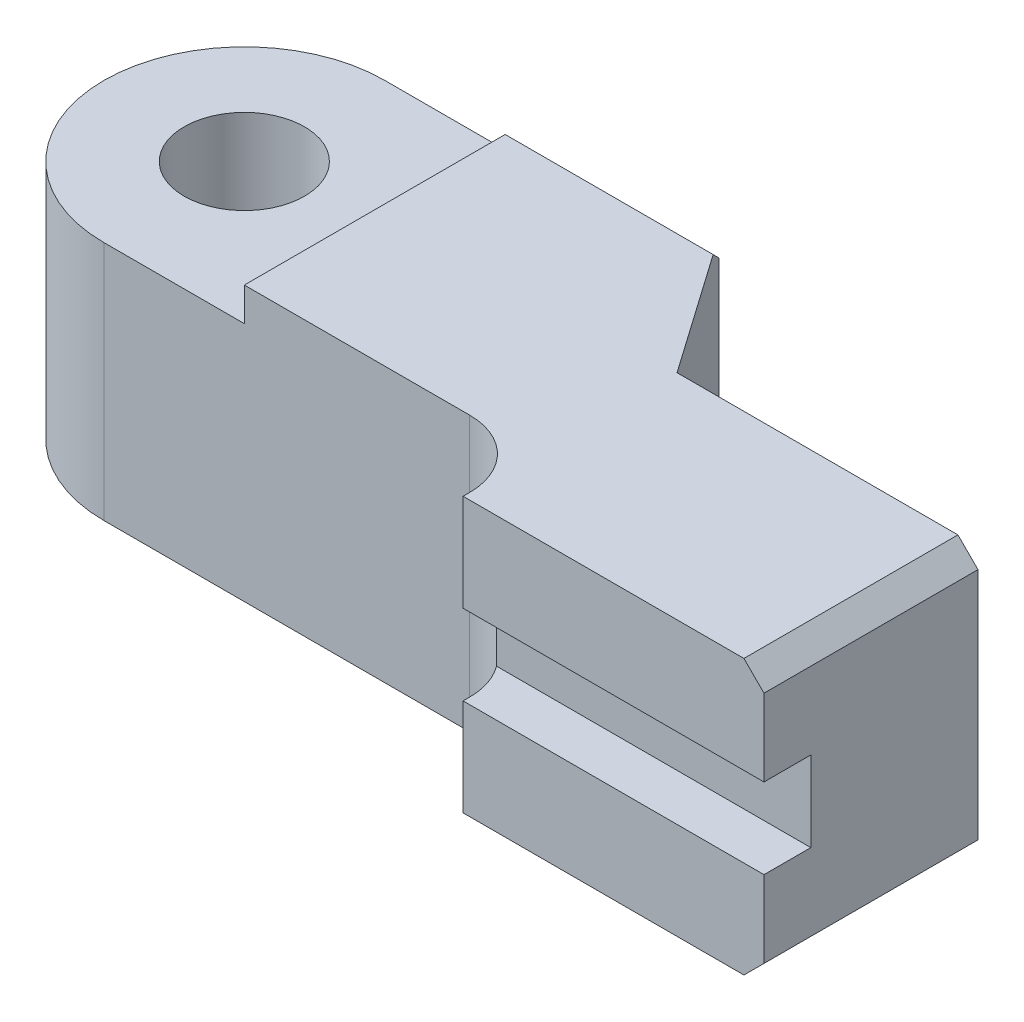
ISO-10303-21;
HEADER;
FILE_DESCRIPTION(('STEP AP214'),'2;1');
FILE_NAME('part.step','',(''),(''),'','','');
FILE_SCHEMA(('AUTOMOTIVE_DESIGN { 1 0 10303 214 1 1 1 1 }'));
ENDSEC;
DATA;
#1=APPLICATION_CONTEXT('core data for automotive mechanical design processes');
#2=APPLICATION_PROTOCOL_DEFINITION('international standard','automotive_design',2000,#1);
#3=PRODUCT_CONTEXT('',#1,'mechanical');
#4=PRODUCT('Part','Part','',(#3));
#5=PRODUCT_RELATED_PRODUCT_CATEGORY('part','',(#4));
#6=PRODUCT_DEFINITION_FORMATION('','',#4);
#7=PRODUCT_DEFINITION_CONTEXT('part definition',#1,'design');
#8=PRODUCT_DEFINITION('design','',#6,#7);
#9=PRODUCT_DEFINITION_SHAPE('','',#8);
#10=(LENGTH_UNIT() NAMED_UNIT(*) SI_UNIT(.MILLI.,.METRE.));
#11=(NAMED_UNIT(*) PLANE_ANGLE_UNIT() SI_UNIT($,.RADIAN.));
#12=(NAMED_UNIT(*) SI_UNIT($,.STERADIAN.) SOLID_ANGLE_UNIT());
#13=UNCERTAINTY_MEASURE_WITH_UNIT(LENGTH_MEASURE(1.E-05),#10,'distance_accuracy_value','');
#14=(GEOMETRIC_REPRESENTATION_CONTEXT(3) GLOBAL_UNCERTAINTY_ASSIGNED_CONTEXT((#13)) GLOBAL_UNIT_ASSIGNED_CONTEXT((#10,
#11,#12)) REPRESENTATION_CONTEXT('',''));
#15=CARTESIAN_POINT('',(0.,0.,0.));
#16=DIRECTION('',(0.,0.,1.));
#17=DIRECTION('',(1.,0.,0.));
#18=AXIS2_PLACEMENT_3D('',#15,#16,#17);
#19=CARTESIAN_POINT('',(54.7043583024038,20.5,0.));
#20=DIRECTION('',(-1.,0.,0.));
#21=DIRECTION('',(0.,0.,1.));
#22=AXIS2_PLACEMENT_3D('',#19,#20,#21);
#23=PLANE('',#22);
#24=DIRECTION('',(0.,-1.,0.));
#25=VECTOR('',#24,1.);
#26=CARTESIAN_POINT('',(54.7043583024038,20.5,32.));
#27=LINE('',#26,#25);
#28=CARTESIAN_POINT('',(54.7043583024038,-6.,32.));
#29=VERTEX_POINT('',#28);
#30=CARTESIAN_POINT('',(54.7043583024038,-17.5,32.));
#31=VERTEX_POINT('',#30);
#32=EDGE_CURVE('E243',#29,#31,#27,.T.);
#33=ORIENTED_EDGE('',*,*,#32,.T.);
#34=DIRECTION('',(0.,0.,-1.));
#35=VECTOR('',#34,1.);
#36=CARTESIAN_POINT('',(54.7043583024038,-17.5,0.));
#37=LINE('',#36,#35);
#38=CARTESIAN_POINT('',(54.7043583024038,-17.5,0.));
#39=VERTEX_POINT('',#38);
#40=EDGE_CURVE('E300',#31,#39,#37,.T.);
#41=ORIENTED_EDGE('',*,*,#40,.T.);
#42=DIRECTION('',(0.,-1.,0.));
#43=VECTOR('',#42,1.);
#44=CARTESIAN_POINT('',(54.7043583024038,20.5,0.));
#45=LINE('',#44,#43);
#46=CARTESIAN_POINT('',(54.7043583024038,17.5,0.));
#47=VERTEX_POINT('',#46);
#48=EDGE_CURVE('E288',#47,#39,#45,.T.);
#49=ORIENTED_EDGE('',*,*,#48,.F.);
#50=DIRECTION('',(0.,0.,1.));
#51=VECTOR('',#50,1.);
#52=CARTESIAN_POINT('',(54.7043583024038,17.5,32.));
#53=LINE('',#52,#51);
#54=CARTESIAN_POINT('',(54.7043583024038,17.5,32.));
#55=VERTEX_POINT('',#54);
#56=EDGE_CURVE('E299',#47,#55,#53,.T.);
#57=ORIENTED_EDGE('',*,*,#56,.T.);
#58=CARTESIAN_POINT('',(54.7043583024038,6.,32.));
#59=VERTEX_POINT('',#58);
#60=EDGE_CURVE('E194',#55,#59,#27,.T.);
#61=ORIENTED_EDGE('',*,*,#60,.T.);
#62=DIRECTION('',(0.,0.,1.));
#63=VECTOR('',#62,1.);
#64=CARTESIAN_POINT('',(54.7043583024038,6.,39.));
#65=LINE('',#64,#63);
#66=CARTESIAN_POINT('',(54.7043583024038,6.,25.));
#67=VERTEX_POINT('',#66);
#68=EDGE_CURVE('E175',#67,#59,#65,.T.);
#69=ORIENTED_EDGE('',*,*,#68,.F.);
#70=DIRECTION('',(0.,1.,0.));
#71=VECTOR('',#70,1.);
#72=CARTESIAN_POINT('',(54.7043583024038,6.,25.));
#73=LINE('',#72,#71);
#74=CARTESIAN_POINT('',(54.7043583024038,-6.,25.));
#75=VERTEX_POINT('',#74);
#76=EDGE_CURVE('E183',#75,#67,#73,.T.);
#77=ORIENTED_EDGE('',*,*,#76,.F.);
#78=DIRECTION('',(0.,0.,-1.));
#79=VECTOR('',#78,1.);
#80=CARTESIAN_POINT('',(54.7043583024038,-6.,39.));
#81=LINE('',#80,#79);
#82=EDGE_CURVE('E185',#29,#75,#81,.T.);
#83=ORIENTED_EDGE('',*,*,#82,.F.);
#84=EDGE_LOOP('',(#33,#41,#49,#57,#61,#69,#77,#83));
#85=FACE_BOUND('',#84,.T.);
#86=ADVANCED_FACE('F41',(#85),#23,.F.);
#87=CARTESIAN_POINT('',(9.70435830240385,20.5,31.0000000000001));
#88=DIRECTION('',(1.,0.,0.));
#89=DIRECTION('',(0.,0.,-1.));
#90=AXIS2_PLACEMENT_3D('',#87,#88,#89);
#91=PLANE('',#90);
#92=DIRECTION('',(0.,-1.,0.));
#93=VECTOR('',#92,1.);
#94=CARTESIAN_POINT('',(9.70435830240385,20.5,32.));
#95=LINE('',#94,#93);
#96=CARTESIAN_POINT('',(9.70435830240385,-6.,32.));
#97=VERTEX_POINT('',#96);
#98=CARTESIAN_POINT('',(9.70435830240385,-20.5,32.));
#99=VERTEX_POINT('',#98);
#100=EDGE_CURVE('E266',#97,#99,#95,.T.);
#101=ORIENTED_EDGE('',*,*,#100,.F.);
#102=DIRECTION('',(0.,0.,-1.));
#103=VECTOR('',#102,1.);
#104=CARTESIAN_POINT('',(9.70435830240385,-6.,31.0000000000001));
#105=LINE('',#104,#103);
#106=CARTESIAN_POINT('',(9.70435830240385,-6.,31.0000000000001));
#107=VERTEX_POINT('',#106);
#108=EDGE_CURVE('E201',#97,#107,#105,.T.);
#109=ORIENTED_EDGE('',*,*,#108,.T.);
#110=DIRECTION('',(0.,-1.,0.));
#111=VECTOR('',#110,1.);
#112=CARTESIAN_POINT('',(9.70435830240385,20.5,31.0000000000001));
#113=LINE('',#112,#111);
#114=CARTESIAN_POINT('',(9.70435830240385,-20.5,31.0000000000001));
#115=VERTEX_POINT('',#114);
#116=EDGE_CURVE('E269',#107,#115,#113,.T.);
#117=ORIENTED_EDGE('',*,*,#116,.T.);
#118=DIRECTION('',(0.,0.,1.));
#119=VECTOR('',#118,1.);
#120=CARTESIAN_POINT('',(9.70435830240385,-20.5,31.0000000000001));
#121=LINE('',#120,#119);
#122=EDGE_CURVE('E257',#115,#99,#121,.T.);
#123=ORIENTED_EDGE('',*,*,#122,.T.);
#124=EDGE_LOOP('',(#101,#109,#117,#123));
#125=FACE_BOUND('',#124,.T.);
#126=ADVANCED_FACE('F362',(#125),#91,.F.);
#127=CARTESIAN_POINT('',(9.70435830240385,20.5,32.));
#128=DIRECTION('',(0.,0.,-1.));
#129=DIRECTION('',(-1.,0.,0.));
#130=AXIS2_PLACEMENT_3D('',#127,#128,#129);
#131=PLANE('',#130);
#132=DIRECTION('',(1.,0.,0.));
#133=VECTOR('',#132,1.);
#134=CARTESIAN_POINT('',(9.70435830240385,-20.5,32.));
#135=LINE('',#134,#133);
#136=CARTESIAN_POINT('',(51.7043583024038,-20.5,32.));
#137=VERTEX_POINT('',#136);
#138=EDGE_CURVE('E235',#99,#137,#135,.T.);
#139=ORIENTED_EDGE('',*,*,#138,.T.);
#140=DIRECTION('',(-0.707106781186547,-0.707106781186548,0.));
#141=VECTOR('',#140,1.);
#142=CARTESIAN_POINT('',(54.7043583024038,-17.5,32.));
#143=LINE('',#142,#141);
#144=EDGE_CURVE('E310',#137,#31,#143,.F.);
#145=ORIENTED_EDGE('',*,*,#144,.T.);
#146=ORIENTED_EDGE('',*,*,#32,.F.);
#147=DIRECTION('',(-1.,0.,0.));
#148=VECTOR('',#147,1.);
#149=CARTESIAN_POINT('',(9.70435830240385,-6.,32.));
#150=LINE('',#149,#148);
#151=EDGE_CURVE('E291',#29,#97,#150,.T.);
#152=ORIENTED_EDGE('',*,*,#151,.T.);
#153=ORIENTED_EDGE('',*,*,#100,.T.);
#154=EDGE_LOOP('',(#139,#145,#146,#152,#153));
#155=FACE_BOUND('',#154,.T.);
#156=ADVANCED_FACE('F369',(#155),#131,.F.);
#157=CARTESIAN_POINT('',(-55.,20.5,21.));
#158=DIRECTION('',(0.,0.,-1.));
#159=DIRECTION('',(-1.,0.,0.));
#160=AXIS2_PLACEMENT_3D('',#157,#158,#159);
#161=PLANE('',#160);
#162=DIRECTION('',(1.,0.,0.));
#163=VECTOR('',#162,1.);
#164=CARTESIAN_POINT('',(-55.,15.5,21.));
#165=LINE('',#164,#163);
#166=CARTESIAN_POINT('',(-55.,15.5,21.));
#167=VERTEX_POINT('',#166);
#168=CARTESIAN_POINT('',(-34.,15.5,21.));
#169=VERTEX_POINT('',#168);
#170=EDGE_CURVE('E215',#167,#169,#165,.T.);
#171=ORIENTED_EDGE('',*,*,#170,.F.);
#172=DIRECTION('',(0.,-1.,0.));
#173=VECTOR('',#172,1.);
#174=CARTESIAN_POINT('',(-55.,20.5,21.));
#175=LINE('',#174,#173);
#176=CARTESIAN_POINT('',(-55.,-20.5,21.));
#177=VERTEX_POINT('',#176);
#178=EDGE_CURVE('E280',#167,#177,#175,.T.);
#179=ORIENTED_EDGE('',*,*,#178,.T.);
#180=DIRECTION('',(1.,0.,0.));
#181=VECTOR('',#180,1.);
#182=CARTESIAN_POINT('',(-55.,-20.5,21.));
#183=LINE('',#182,#181);
#184=CARTESIAN_POINT('',(-0.295641697596222,-20.5,21.));
#185=VERTEX_POINT('',#184);
#186=EDGE_CURVE('E254',#177,#185,#183,.T.);
#187=ORIENTED_EDGE('',*,*,#186,.T.);
#188=DIRECTION('',(0.,-1.,0.));
#189=VECTOR('',#188,1.);
#190=CARTESIAN_POINT('',(-0.295641697596222,20.5,21.));
#191=LINE('',#190,#189);
#192=CARTESIAN_POINT('',(-0.295641697596222,20.5,21.));
#193=VERTEX_POINT('',#192);
#194=EDGE_CURVE('E273',#193,#185,#191,.T.);
#195=ORIENTED_EDGE('',*,*,#194,.F.);
#196=DIRECTION('',(1.,0.,0.));
#197=VECTOR('',#196,1.);
#198=CARTESIAN_POINT('',(-55.,20.5,21.));
#199=LINE('',#198,#197);
#200=CARTESIAN_POINT('',(-34.,20.5,21.));
#201=VERTEX_POINT('',#200);
#202=EDGE_CURVE('E232',#201,#193,#199,.T.);
#203=ORIENTED_EDGE('',*,*,#202,.F.);
#204=DIRECTION('',(0.,1.,0.));
#205=VECTOR('',#204,1.);
#206=CARTESIAN_POINT('',(-34.,15.5,21.));
#207=LINE('',#206,#205);
#208=EDGE_CURVE('E218',#169,#201,#207,.T.);
#209=ORIENTED_EDGE('',*,*,#208,.F.);
#210=EDGE_LOOP('',(#171,#179,#187,#195,#203,#209));
#211=FACE_BOUND('',#210,.T.);
#212=ADVANCED_FACE('F425',(#211),#161,.F.);
#213=CARTESIAN_POINT('',(-55.,20.5,0.));
#214=DIRECTION('',(0.,-1.,0.));
#215=DIRECTION('',(0.,0.,-1.));
#216=AXIS2_PLACEMENT_3D('',#213,#214,#215);
#217=CYLINDRICAL_SURFACE('',#216,21.);
#218=CARTESIAN_POINT('',(-55.,15.5,0.));
#219=DIRECTION('',(0.,1.,0.));
#220=DIRECTION('',(0.,0.,1.));
#221=AXIS2_PLACEMENT_3D('',#218,#219,#220);
#222=CIRCLE('',#221,21.);
#223=CARTESIAN_POINT('',(-55.,15.5,-21.));
#224=VERTEX_POINT('',#223);
#225=EDGE_CURVE('E209',#224,#167,#222,.T.);
#226=ORIENTED_EDGE('',*,*,#225,.F.);
#227=DIRECTION('',(0.,-1.,0.));
#228=VECTOR('',#227,1.);
#229=CARTESIAN_POINT('',(-55.,20.5,-21.));
#230=LINE('',#229,#228);
#231=CARTESIAN_POINT('',(-55.,-20.5,-21.));
#232=VERTEX_POINT('',#231);
#233=EDGE_CURVE('E276',#224,#232,#230,.T.);
#234=ORIENTED_EDGE('',*,*,#233,.T.);
#235=CARTESIAN_POINT('',(-55.,-20.5,0.));
#236=DIRECTION('',(0.,1.,0.));
#237=DIRECTION('',(0.,0.,1.));
#238=AXIS2_PLACEMENT_3D('',#235,#236,#237);
#239=CIRCLE('',#238,21.);
#240=EDGE_CURVE('E252',#232,#177,#239,.T.);
#241=ORIENTED_EDGE('',*,*,#240,.T.);
#242=ORIENTED_EDGE('',*,*,#178,.F.);
#243=EDGE_LOOP('',(#226,#234,#241,#242));
#244=FACE_BOUND('',#243,.T.);
#245=ADVANCED_FACE('F407',(#244),#217,.T.);
#246=CARTESIAN_POINT('',(-55.,20.5,0.));
#247=DIRECTION('',(0.,-1.,0.));
#248=DIRECTION('',(0.,0.,-1.));
#249=AXIS2_PLACEMENT_3D('',#246,#247,#248);
#250=CYLINDRICAL_SURFACE('',#249,9.);
#251=CARTESIAN_POINT('',(-55.,-20.5,0.));
#252=DIRECTION('',(0.,1.,0.));
#253=DIRECTION('',(0.,0.,1.));
#254=AXIS2_PLACEMENT_3D('',#251,#252,#253);
#255=CIRCLE('',#254,9.);
#256=CARTESIAN_POINT('',(-55.,-20.5,8.99999999999999));
#257=VERTEX_POINT('',#256);
#258=EDGE_CURVE('E223',#257,#257,#255,.T.);
#259=ORIENTED_EDGE('',*,*,#258,.F.);
#260=EDGE_LOOP('',(#259));
#261=FACE_BOUND('',#260,.T.);
#262=CARTESIAN_POINT('',(-55.,15.5,0.));
#263=DIRECTION('',(0.,1.,0.));
#264=DIRECTION('',(0.,0.,1.));
#265=AXIS2_PLACEMENT_3D('',#262,#263,#264);
#266=CIRCLE('',#265,9.);
#267=CARTESIAN_POINT('',(-55.,15.5,8.99999999999999));
#268=VERTEX_POINT('',#267);
#269=EDGE_CURVE('E224',#268,#268,#266,.T.);
#270=ORIENTED_EDGE('',*,*,#269,.T.);
#271=EDGE_LOOP('',(#270));
#272=FACE_BOUND('',#271,.T.);
#273=ADVANCED_FACE('F404',(#261,#272),#250,.F.);
#274=CARTESIAN_POINT('',(-0.295641697596152,20.5,31.));
#275=DIRECTION('',(0.,1.,0.));
#276=DIRECTION('',(0.,0.,1.));
#277=AXIS2_PLACEMENT_3D('',#274,#275,#276);
#278=PLANE('',#277);
#279=DIRECTION('',(1.,0.,0.));
#280=VECTOR('',#279,1.);
#281=CARTESIAN_POINT('',(9.70435830240385,20.5,32.));
#282=LINE('',#281,#280);
#283=CARTESIAN_POINT('',(9.70435830240385,20.5,32.));
#284=VERTEX_POINT('',#283);
#285=CARTESIAN_POINT('',(51.7043583024039,20.5,32.));
#286=VERTEX_POINT('',#285);
#287=EDGE_CURVE('E241',#284,#286,#282,.T.);
#288=ORIENTED_EDGE('',*,*,#287,.T.);
#289=DIRECTION('',(0.,0.,-1.));
#290=VECTOR('',#289,1.);
#291=CARTESIAN_POINT('',(51.7043583024039,20.5,0.));
#292=LINE('',#291,#290);
#293=CARTESIAN_POINT('',(51.7043583024039,20.5,0.));
#294=VERTEX_POINT('',#293);
#295=EDGE_CURVE('E314',#286,#294,#292,.T.);
#296=ORIENTED_EDGE('',*,*,#295,.T.);
#297=DIRECTION('',(-1.,0.,0.));
#298=VECTOR('',#297,1.);
#299=CARTESIAN_POINT('',(54.7043583024038,20.5,0.));
#300=LINE('',#299,#298);
#301=CARTESIAN_POINT('',(9.70435830240384,20.5,0.));
#302=VERTEX_POINT('',#301);
#303=EDGE_CURVE('E228',#294,#302,#300,.T.);
#304=ORIENTED_EDGE('',*,*,#303,.T.);
#305=DIRECTION('',(-0.573576436351043,0.,-0.819152044288994));
#306=VECTOR('',#305,1.);
#307=CARTESIAN_POINT('',(-4.99999999999999,20.5,-21.0000000000001));
#308=LINE('',#307,#306);
#309=CARTESIAN_POINT('',(-2.89937738537089,20.5,-18.0000000000001));
#310=VERTEX_POINT('',#309);
#311=EDGE_CURVE('E233',#302,#310,#308,.T.);
#312=ORIENTED_EDGE('',*,*,#311,.T.);
#313=DIRECTION('',(-1.,0.,0.));
#314=VECTOR('',#313,1.);
#315=CARTESIAN_POINT('',(-34.,20.5,-18.));
#316=LINE('',#315,#314);
#317=CARTESIAN_POINT('',(-34.,20.5,-18.));
#318=VERTEX_POINT('',#317);
#319=EDGE_CURVE('E313',#310,#318,#316,.T.);
#320=ORIENTED_EDGE('',*,*,#319,.T.);
#321=DIRECTION('',(0.,0.,-1.));
#322=VECTOR('',#321,1.);
#323=CARTESIAN_POINT('',(-34.,20.5,-21.0000000000001));
#324=LINE('',#323,#322);
#325=EDGE_CURVE('E207',#201,#318,#324,.T.);
#326=ORIENTED_EDGE('',*,*,#325,.F.);
#327=ORIENTED_EDGE('',*,*,#202,.T.);
#328=CARTESIAN_POINT('',(-0.295641697596152,20.5,31.));
#329=DIRECTION('',(0.,-1.,0.));
#330=DIRECTION('',(0.,0.,1.));
#331=AXIS2_PLACEMENT_3D('',#328,#329,#330);
#332=CIRCLE('',#331,10.);
#333=CARTESIAN_POINT('',(9.70435830240385,20.5,31.0000000000001));
#334=VERTEX_POINT('',#333);
#335=EDGE_CURVE('E240',#193,#334,#332,.T.);
#336=ORIENTED_EDGE('',*,*,#335,.T.);
#337=DIRECTION('',(0.,0.,1.));
#338=VECTOR('',#337,1.);
#339=CARTESIAN_POINT('',(9.70435830240385,20.5,31.0000000000001));
#340=LINE('',#339,#338);
#341=EDGE_CURVE('E239',#334,#284,#340,.T.);
#342=ORIENTED_EDGE('',*,*,#341,.T.);
#343=EDGE_LOOP('',(#288,#296,#304,#312,#320,#326,#327,#336,#342));
#344=FACE_BOUND('',#343,.T.);
#345=ADVANCED_FACE('F330',(#344),#278,.T.);
#346=CARTESIAN_POINT('',(-0.295641697596152,-20.5,31.));
#347=DIRECTION('',(0.,1.,0.));
#348=DIRECTION('',(0.,0.,1.));
#349=AXIS2_PLACEMENT_3D('',#346,#347,#348);
#350=PLANE('',#349);
#351=DIRECTION('',(-1.,0.,0.));
#352=VECTOR('',#351,1.);
#353=CARTESIAN_POINT('',(54.7043583024038,-20.5,0.));
#354=LINE('',#353,#352);
#355=CARTESIAN_POINT('',(51.7043583024038,-20.5,0.));
#356=VERTEX_POINT('',#355);
#357=CARTESIAN_POINT('',(9.70435830240384,-20.5,0.));
#358=VERTEX_POINT('',#357);
#359=EDGE_CURVE('E229',#356,#358,#354,.T.);
#360=ORIENTED_EDGE('',*,*,#359,.F.);
#361=DIRECTION('',(0.,0.,1.));
#362=VECTOR('',#361,1.);
#363=CARTESIAN_POINT('',(51.7043583024039,-20.5,31.));
#364=LINE('',#363,#362);
#365=EDGE_CURVE('E307',#356,#137,#364,.T.);
#366=ORIENTED_EDGE('',*,*,#365,.T.);
#367=ORIENTED_EDGE('',*,*,#138,.F.);
#368=ORIENTED_EDGE('',*,*,#122,.F.);
#369=CARTESIAN_POINT('',(-0.295641697596152,-20.5,31.));
#370=DIRECTION('',(0.,-1.,0.));
#371=DIRECTION('',(0.,0.,1.));
#372=AXIS2_PLACEMENT_3D('',#369,#370,#371);
#373=CIRCLE('',#372,10.);
#374=EDGE_CURVE('E260',#185,#115,#373,.T.);
#375=ORIENTED_EDGE('',*,*,#374,.F.);
#376=ORIENTED_EDGE('',*,*,#186,.F.);
#377=ORIENTED_EDGE('',*,*,#240,.F.);
#378=DIRECTION('',(-1.,0.,0.));
#379=VECTOR('',#378,1.);
#380=CARTESIAN_POINT('',(-55.,-20.5,-21.));
#381=LINE('',#380,#379);
#382=CARTESIAN_POINT('',(-4.99999999999999,-20.5,-21.0000000000001));
#383=VERTEX_POINT('',#382);
#384=EDGE_CURVE('E249',#383,#232,#381,.T.);
#385=ORIENTED_EDGE('',*,*,#384,.F.);
#386=DIRECTION('',(-0.573576436351043,0.,-0.819152044288994));
#387=VECTOR('',#386,1.);
#388=CARTESIAN_POINT('',(-4.99999999999999,-20.5,-21.0000000000001));
#389=LINE('',#388,#387);
#390=EDGE_CURVE('E248',#358,#383,#389,.T.);
#391=ORIENTED_EDGE('',*,*,#390,.F.);
#392=EDGE_LOOP('',(#360,#366,#367,#368,#375,#376,#377,#385,#391));
#393=FACE_BOUND('',#392,.T.);
#394=ORIENTED_EDGE('',*,*,#258,.T.);
#395=EDGE_LOOP('',(#394));
#396=FACE_BOUND('',#395,.T.);
#397=ADVANCED_FACE('F342',(#393,#396),#350,.F.);
#398=CARTESIAN_POINT('',(54.7043583024038,20.5,0.));
#399=DIRECTION('',(0.,0.,1.));
#400=DIRECTION('',(1.,0.,0.));
#401=AXIS2_PLACEMENT_3D('',#398,#399,#400);
#402=PLANE('',#401);
#403=ORIENTED_EDGE('',*,*,#48,.T.);
#404=DIRECTION('',(0.707106781186547,0.707106781186548,0.));
#405=VECTOR('',#404,1.);
#406=CARTESIAN_POINT('',(54.7043583024038,-17.5,0.));
#407=LINE('',#406,#405);
#408=EDGE_CURVE('E302',#39,#356,#407,.F.);
#409=ORIENTED_EDGE('',*,*,#408,.T.);
#410=ORIENTED_EDGE('',*,*,#359,.T.);
#411=DIRECTION('',(0.,-1.,0.));
#412=VECTOR('',#411,1.);
#413=CARTESIAN_POINT('',(9.70435830240384,20.5,0.));
#414=LINE('',#413,#412);
#415=EDGE_CURVE('E284',#302,#358,#414,.T.);
#416=ORIENTED_EDGE('',*,*,#415,.F.);
#417=ORIENTED_EDGE('',*,*,#303,.F.);
#418=DIRECTION('',(0.707106781186545,-0.70710678118655,0.));
#419=VECTOR('',#418,1.);
#420=CARTESIAN_POINT('',(51.7043583024039,20.5,0.));
#421=LINE('',#420,#419);
#422=EDGE_CURVE('E301',#294,#47,#421,.T.);
#423=ORIENTED_EDGE('',*,*,#422,.T.);
#424=EDGE_LOOP('',(#403,#409,#410,#416,#417,#423));
#425=FACE_BOUND('',#424,.T.);
#426=ADVANCED_FACE('F331',(#425),#402,.F.);
#427=CARTESIAN_POINT('',(-4.99999999999999,20.5,-21.0000000000001));
#428=DIRECTION('',(-0.819152044288994,0.,0.573576436351043));
#429=DIRECTION('',(0.573576436351043,0.,0.819152044288994));
#430=AXIS2_PLACEMENT_3D('',#427,#428,#429);
#431=PLANE('',#430);
#432=DIRECTION('',(0.,-1.,0.));
#433=VECTOR('',#432,1.);
#434=CARTESIAN_POINT('',(-4.99999999999999,20.5,-21.0000000000001));
#435=LINE('',#434,#433);
#436=CARTESIAN_POINT('',(-4.99999999999999,17.5,-21.0000000000001));
#437=VERTEX_POINT('',#436);
#438=EDGE_CURVE('E281',#437,#383,#435,.T.);
#439=ORIENTED_EDGE('',*,*,#438,.F.);
#440=DIRECTION('',(0.443712606279655,0.633687274224643,0.633687274224643));
#441=VECTOR('',#440,1.);
#442=CARTESIAN_POINT('',(-2.38675161975986,21.2321054653621,-17.267894534638));
#443=LINE('',#442,#441);
#444=EDGE_CURVE('E11',#437,#310,#443,.T.);
#445=ORIENTED_EDGE('',*,*,#444,.T.);
#446=ORIENTED_EDGE('',*,*,#311,.F.);
#447=ORIENTED_EDGE('',*,*,#415,.T.);
#448=ORIENTED_EDGE('',*,*,#390,.T.);
#449=EDGE_LOOP('',(#439,#445,#446,#447,#448));
#450=FACE_BOUND('',#449,.T.);
#451=ADVANCED_FACE('F351',(#450),#431,.F.);
#452=CARTESIAN_POINT('',(-55.,20.5,-21.));
#453=DIRECTION('',(0.,0.,1.));
#454=DIRECTION('',(1.,0.,0.));
#455=AXIS2_PLACEMENT_3D('',#452,#453,#454);
#456=PLANE('',#455);
#457=DIRECTION('',(0.,1.,0.));
#458=VECTOR('',#457,1.);
#459=CARTESIAN_POINT('',(-34.,15.5,-21.0000000000001));
#460=LINE('',#459,#458);
#461=CARTESIAN_POINT('',(-34.,15.5,-21.0000000000001));
#462=VERTEX_POINT('',#461);
#463=CARTESIAN_POINT('',(-34.,17.5,-21.0000000000001));
#464=VERTEX_POINT('',#463);
#465=EDGE_CURVE('E222',#462,#464,#460,.T.);
#466=ORIENTED_EDGE('',*,*,#465,.T.);
#467=DIRECTION('',(1.,0.,0.));
#468=VECTOR('',#467,1.);
#469=CARTESIAN_POINT('',(-4.99999999999999,17.5,-21.0000000000001));
#470=LINE('',#469,#468);
#471=EDGE_CURVE('E49',#464,#437,#470,.T.);
#472=ORIENTED_EDGE('',*,*,#471,.T.);
#473=ORIENTED_EDGE('',*,*,#438,.T.);
#474=ORIENTED_EDGE('',*,*,#384,.T.);
#475=ORIENTED_EDGE('',*,*,#233,.F.);
#476=DIRECTION('',(-1.,0.,0.));
#477=VECTOR('',#476,1.);
#478=CARTESIAN_POINT('',(-34.,15.5,-21.0000000000001));
#479=LINE('',#478,#477);
#480=EDGE_CURVE('E220',#462,#224,#479,.T.);
#481=ORIENTED_EDGE('',*,*,#480,.F.);
#482=EDGE_LOOP('',(#466,#472,#473,#474,#475,#481));
#483=FACE_BOUND('',#482,.T.);
#484=ADVANCED_FACE('F419',(#483),#456,.F.);
#485=CARTESIAN_POINT('',(-0.295641697596152,20.5,31.));
#486=DIRECTION('',(0.,-1.,0.));
#487=DIRECTION('',(0.,0.,-1.));
#488=AXIS2_PLACEMENT_3D('',#485,#486,#487);
#489=CYLINDRICAL_SURFACE('',#488,10.);
#490=ORIENTED_EDGE('',*,*,#116,.F.);
#491=CARTESIAN_POINT('',(-0.295641697596152,-6.,31.));
#492=DIRECTION('',(0.,-1.,0.));
#493=DIRECTION('',(0.,0.,-1.));
#494=AXIS2_PLACEMENT_3D('',#491,#492,#493);
#495=CIRCLE('',#494,10.);
#496=CARTESIAN_POINT('',(7.70435830240387,-6.,25.));
#497=VERTEX_POINT('',#496);
#498=EDGE_CURVE('E206',#107,#497,#495,.F.);
#499=ORIENTED_EDGE('',*,*,#498,.T.);
#500=DIRECTION('',(0.,-1.,0.));
#501=VECTOR('',#500,1.);
#502=CARTESIAN_POINT('',(7.70435830240387,20.5,25.));
#503=LINE('',#502,#501);
#504=CARTESIAN_POINT('',(7.70435830240387,6.,25.));
#505=VERTEX_POINT('',#504);
#506=EDGE_CURVE('E296',#497,#505,#503,.F.);
#507=ORIENTED_EDGE('',*,*,#506,.T.);
#508=CARTESIAN_POINT('',(-0.295641697596152,6.,31.));
#509=DIRECTION('',(0.,1.,0.));
#510=DIRECTION('',(0.,0.,1.));
#511=AXIS2_PLACEMENT_3D('',#508,#509,#510);
#512=CIRCLE('',#511,10.);
#513=CARTESIAN_POINT('',(9.70435830240385,6.,31.0000000000001));
#514=VERTEX_POINT('',#513);
#515=EDGE_CURVE('E176',#505,#514,#512,.F.);
#516=ORIENTED_EDGE('',*,*,#515,.T.);
#517=EDGE_CURVE('E271',#334,#514,#113,.T.);
#518=ORIENTED_EDGE('',*,*,#517,.F.);
#519=ORIENTED_EDGE('',*,*,#335,.F.);
#520=ORIENTED_EDGE('',*,*,#194,.T.);
#521=ORIENTED_EDGE('',*,*,#374,.T.);
#522=EDGE_LOOP('',(#490,#499,#507,#516,#518,#519,#520,#521));
#523=FACE_BOUND('',#522,.T.);
#524=ADVANCED_FACE('F418',(#523),#489,.F.);
#525=ORIENTED_EDGE('',*,*,#517,.T.);
#526=DIRECTION('',(0.,0.,1.));
#527=VECTOR('',#526,1.);
#528=CARTESIAN_POINT('',(9.70435830240385,6.,31.0000000000001));
#529=LINE('',#528,#527);
#530=CARTESIAN_POINT('',(9.70435830240385,6.,32.));
#531=VERTEX_POINT('',#530);
#532=EDGE_CURVE('E196',#514,#531,#529,.T.);
#533=ORIENTED_EDGE('',*,*,#532,.T.);
#534=EDGE_CURVE('E270',#284,#531,#95,.T.);
#535=ORIENTED_EDGE('',*,*,#534,.F.);
#536=ORIENTED_EDGE('',*,*,#341,.F.);
#537=EDGE_LOOP('',(#525,#533,#535,#536));
#538=FACE_BOUND('',#537,.T.);
#539=ADVANCED_FACE('F375',(#538),#91,.F.);
#540=ORIENTED_EDGE('',*,*,#60,.F.);
#541=DIRECTION('',(-0.707106781186545,0.70710678118655,0.));
#542=VECTOR('',#541,1.);
#543=CARTESIAN_POINT('',(51.7043583024039,20.5,32.));
#544=LINE('',#543,#542);
#545=EDGE_CURVE('E320',#55,#286,#544,.T.);
#546=ORIENTED_EDGE('',*,*,#545,.T.);
#547=ORIENTED_EDGE('',*,*,#287,.F.);
#548=ORIENTED_EDGE('',*,*,#534,.T.);
#549=DIRECTION('',(1.,0.,0.));
#550=VECTOR('',#549,1.);
#551=CARTESIAN_POINT('',(9.70435830240385,6.,32.));
#552=LINE('',#551,#550);
#553=EDGE_CURVE('E289',#531,#59,#552,.T.);
#554=ORIENTED_EDGE('',*,*,#553,.T.);
#555=EDGE_LOOP('',(#540,#546,#547,#548,#554));
#556=FACE_BOUND('',#555,.T.);
#557=ADVANCED_FACE('F325',(#556),#131,.F.);
#558=CARTESIAN_POINT('',(-34.,15.5,-21.0000000000001));
#559=DIRECTION('',(1.,0.,0.));
#560=DIRECTION('',(0.,0.,-1.));
#561=AXIS2_PLACEMENT_3D('',#558,#559,#560);
#562=PLANE('',#561);
#563=ORIENTED_EDGE('',*,*,#325,.T.);
#564=DIRECTION('',(0.,-0.707106781186548,-0.707106781186547));
#565=VECTOR('',#564,1.);
#566=CARTESIAN_POINT('',(-34.,20.5,-18.0000000000001));
#567=LINE('',#566,#565);
#568=EDGE_CURVE('E63',#318,#464,#567,.T.);
#569=ORIENTED_EDGE('',*,*,#568,.T.);
#570=ORIENTED_EDGE('',*,*,#465,.F.);
#571=DIRECTION('',(0.,0.,-1.));
#572=VECTOR('',#571,1.);
#573=CARTESIAN_POINT('',(-34.,15.5,-21.0000000000001));
#574=LINE('',#573,#572);
#575=EDGE_CURVE('E212',#169,#462,#574,.T.);
#576=ORIENTED_EDGE('',*,*,#575,.F.);
#577=ORIENTED_EDGE('',*,*,#208,.T.);
#578=EDGE_LOOP('',(#563,#569,#570,#576,#577));
#579=FACE_BOUND('',#578,.T.);
#580=ADVANCED_FACE('F402',(#579),#562,.F.);
#581=CARTESIAN_POINT('',(-55.,15.5,0.));
#582=DIRECTION('',(0.,1.,0.));
#583=DIRECTION('',(0.,0.,1.));
#584=AXIS2_PLACEMENT_3D('',#581,#582,#583);
#585=PLANE('',#584);
#586=ORIENTED_EDGE('',*,*,#269,.F.);
#587=EDGE_LOOP('',(#586));
#588=FACE_BOUND('',#587,.T.);
#589=ORIENTED_EDGE('',*,*,#225,.T.);
#590=ORIENTED_EDGE('',*,*,#170,.T.);
#591=ORIENTED_EDGE('',*,*,#575,.T.);
#592=ORIENTED_EDGE('',*,*,#480,.T.);
#593=EDGE_LOOP('',(#589,#590,#591,#592));
#594=FACE_BOUND('',#593,.T.);
#595=ADVANCED_FACE('F396',(#588,#594),#585,.T.);
#596=CARTESIAN_POINT('',(-20.2956416975961,6.,25.));
#597=DIRECTION('',(0.,0.,-1.));
#598=DIRECTION('',(-1.,0.,0.));
#599=AXIS2_PLACEMENT_3D('',#596,#597,#598);
#600=PLANE('',#599);
#601=DIRECTION('',(1.,0.,0.));
#602=VECTOR('',#601,1.);
#603=CARTESIAN_POINT('',(-20.2956416975961,-6.,25.));
#604=LINE('',#603,#602);
#605=EDGE_CURVE('E182',#497,#75,#604,.T.);
#606=ORIENTED_EDGE('',*,*,#605,.T.);
#607=ORIENTED_EDGE('',*,*,#76,.T.);
#608=DIRECTION('',(1.,0.,0.));
#609=VECTOR('',#608,1.);
#610=CARTESIAN_POINT('',(-20.2956416975961,6.,25.));
#611=LINE('',#610,#609);
#612=EDGE_CURVE('E171',#505,#67,#611,.T.);
#613=ORIENTED_EDGE('',*,*,#612,.F.);
#614=ORIENTED_EDGE('',*,*,#506,.F.);
#615=EDGE_LOOP('',(#606,#607,#613,#614));
#616=FACE_BOUND('',#615,.T.);
#617=ADVANCED_FACE('F186',(#616),#600,.F.);
#618=CARTESIAN_POINT('',(-20.2956416975961,-6.,39.));
#619=DIRECTION('',(0.,-1.,0.));
#620=DIRECTION('',(0.,0.,-1.));
#621=AXIS2_PLACEMENT_3D('',#618,#619,#620);
#622=PLANE('',#621);
#623=ORIENTED_EDGE('',*,*,#108,.F.);
#624=ORIENTED_EDGE('',*,*,#151,.F.);
#625=ORIENTED_EDGE('',*,*,#82,.T.);
#626=ORIENTED_EDGE('',*,*,#605,.F.);
#627=ORIENTED_EDGE('',*,*,#498,.F.);
#628=EDGE_LOOP('',(#623,#624,#625,#626,#627));
#629=FACE_BOUND('',#628,.T.);
#630=ADVANCED_FACE('F389',(#629),#622,.F.);
#631=CARTESIAN_POINT('',(-20.2956416975961,6.,39.));
#632=DIRECTION('',(0.,1.,0.));
#633=DIRECTION('',(0.,0.,1.));
#634=AXIS2_PLACEMENT_3D('',#631,#632,#633);
#635=PLANE('',#634);
#636=ORIENTED_EDGE('',*,*,#612,.T.);
#637=ORIENTED_EDGE('',*,*,#68,.T.);
#638=ORIENTED_EDGE('',*,*,#553,.F.);
#639=ORIENTED_EDGE('',*,*,#532,.F.);
#640=ORIENTED_EDGE('',*,*,#515,.F.);
#641=EDGE_LOOP('',(#636,#637,#638,#639,#640));
#642=FACE_BOUND('',#641,.T.);
#643=ADVANCED_FACE('F174',(#642),#635,.F.);
#644=CARTESIAN_POINT('',(54.7043583024038,-17.5,0.));
#645=DIRECTION('',(-0.707106781186548,0.707106781186547,0.));
#646=DIRECTION('',(0.,0.,-1.));
#647=AXIS2_PLACEMENT_3D('',#644,#645,#646);
#648=PLANE('',#647);
#649=ORIENTED_EDGE('',*,*,#144,.F.);
#650=ORIENTED_EDGE('',*,*,#365,.F.);
#651=ORIENTED_EDGE('',*,*,#408,.F.);
#652=ORIENTED_EDGE('',*,*,#40,.F.);
#653=EDGE_LOOP('',(#649,#650,#651,#652));
#654=FACE_BOUND('',#653,.T.);
#655=ADVANCED_FACE('F340',(#654),#648,.F.);
#656=CARTESIAN_POINT('',(51.7043583024039,20.5,31.));
#657=DIRECTION('',(0.70710678118655,0.707106781186545,0.));
#658=DIRECTION('',(0.,0.,1.));
#659=AXIS2_PLACEMENT_3D('',#656,#657,#658);
#660=PLANE('',#659);
#661=ORIENTED_EDGE('',*,*,#545,.F.);
#662=ORIENTED_EDGE('',*,*,#56,.F.);
#663=ORIENTED_EDGE('',*,*,#422,.F.);
#664=ORIENTED_EDGE('',*,*,#295,.F.);
#665=EDGE_LOOP('',(#661,#662,#663,#664));
#666=FACE_BOUND('',#665,.T.);
#667=ADVANCED_FACE('F332',(#666),#660,.T.);
#668=CARTESIAN_POINT('',(-0.295641697596213,20.5,-18.0000000000001));
#669=DIRECTION('',(0.,0.707106781186547,-0.707106781186548));
#670=DIRECTION('',(1.,0.,0.));
#671=AXIS2_PLACEMENT_3D('',#668,#669,#670);
#672=PLANE('',#671);
#673=ORIENTED_EDGE('',*,*,#444,.F.);
#674=ORIENTED_EDGE('',*,*,#471,.F.);
#675=ORIENTED_EDGE('',*,*,#568,.F.);
#676=ORIENTED_EDGE('',*,*,#319,.F.);
#677=EDGE_LOOP('',(#673,#674,#675,#676));
#678=FACE_BOUND('',#677,.T.);
#679=ADVANCED_FACE('F42',(#678),#672,.T.);
#680=CLOSED_SHELL('',(#86,#126,#156,#212,#245,#273,#345,#397,#426,#451,#484,#524,#539,#557,#580,
#595,#617,#630,#643,#655,#667,#679));
#681=MANIFOLD_SOLID_BREP('B2',#680);
#682=ADVANCED_BREP_SHAPE_REPRESENTATION('',(#18,#681),#14);
#683=SHAPE_DEFINITION_REPRESENTATION(#9,#682);
ENDSEC;
END-ISO-10303-21;
